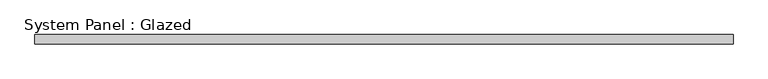
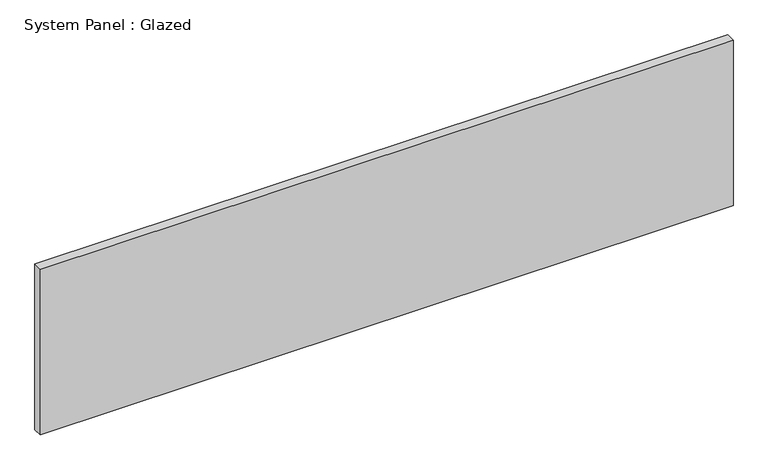
"""IFC4 building model written with IfcOpenShell, lengths in millimetres: plate geometry, System Panel : Glazed."""

from ifc_helpers import new_model, si_unit, origin, origin_with_axes, place, context, project, spatial, polyline, outline, extrude, source, transform, mapped, element, save


def system_panel_glazed_df97d9fa(model_context):
    return source(origin(), model_context, "Body", "SweptSolid", [
        extrude(outline(polyline([(950.7907705, 19.05), (-950.7907705, 19.05), (-950.7907705, 44.45), (950.7907705, 44.45), (950.7907705, 19.05)])), origin_with_axes(), (0.0, 0.0, 1.0), 481.0119748),
    ])


if __name__ == "__main__":
    model = new_model("IFC4")
    model_context = context("Model", 3, world=origin())
    ifc_project = project(units=[si_unit("LENGTHUNIT", "METRE", prefix="MILLI")], contexts=[model_context])
    site = spatial("IfcSite", under=ifc_project)
    building = spatial("IfcBuilding", under=site)
    placement = place(None, origin())
    system_panel_glazed_shape = system_panel_glazed_df97d9fa(model_context)
    element("IfcPlate", 1, ObjectType="System Panel : Glazed", at=placement, inside=building, context=model_context, shape_type="MappedRepresentation", body=[
        mapped(system_panel_glazed_shape, transform((0.0, 0.0, 0.0), x_axis=(1.0, 0.0, 0.0), y_axis=(0.0, 1.0, 0.0), z_axis=(0.0, 0.0, 1.0))),
    ])
    save(model, "model.ifc")

# Revit data of these elements
# Type "System Panel : Glazed"
#   Construction Type Id = "GSP4R"
#   Analytic Construction = "1/8 in Pilkington single glazing"
#   Visual Light Transmittance = 0.9
#   Solar Heat Gain Coefficient = 0.86
#   Heat Transfer Coefficient (U) = 1.18115 BTU/(h·ft²·°F)
#   Define Thermal Properties by = 1
# Element 1 (IfcPlate, "System Panel : Glazed")
#   Materials on its faces: "Glass"
# Materials
#   "Glass": class "Glass", colour RGB 0 128 192, transparency 0.75, Description = "Soda Lime Glass", Cost = 0
